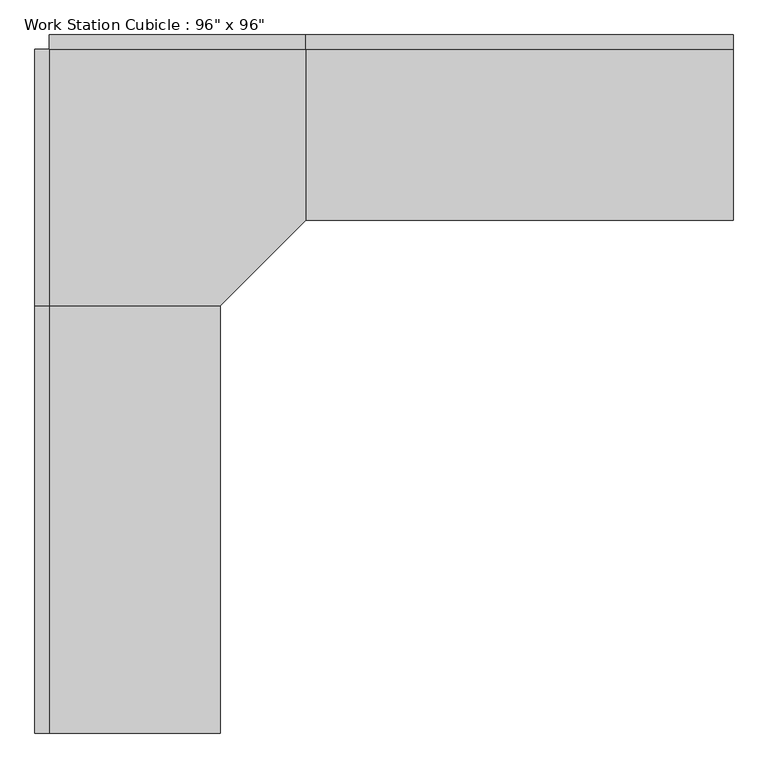
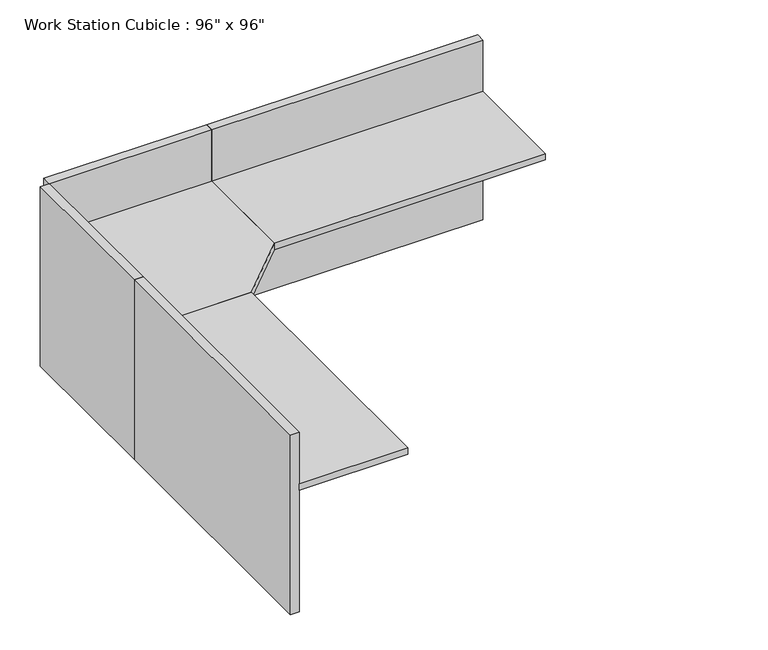
"""IFC4 building model written with IfcOpenShell, lengths in millimetres: furniture geometry."""

from ifc_helpers import new_model, si_unit, frame, origin, origin_with_axes, place, context, project, spatial, polyline, outline, extrude, source, transform, mapped, element, save


def furniture_b89246da(model_context):
    return source(origin(), model_context, "Body", "SweptSolid", [
        extrude(outline(polyline([(-80.9317522, -545.8230076), (833.4682478, -545.8230076), (833.4682478, -1155.4230076), (528.6682478, -1460.2230076), (-80.9317522, -1460.2230076), (-80.9317522, -545.8230076)])), frame((0.0, 0.0, 723.9), z_axis=(0.0, 0.0, 1.0), x_axis=(1.0, 0.0, 0.0)), (0.0, 0.0, 1.0), 38.1),
        extrude(outline(polyline([(528.6682478, -2984.2230076), (-80.9317522, -2984.2230076), (-80.9317522, -1460.2230076), (528.6682478, -1460.2230076), (528.6682478, -2984.2230076)])), frame((0.0, 0.0, 723.9), z_axis=(0.0, 0.0, 1.0), x_axis=(1.0, 0.0, 0.0)), (0.0, 0.0, 1.0), 38.1),
        extrude(outline(polyline([(2357.4682478, -1155.4230076), (833.4682478, -1155.4230076), (833.4682478, -545.8230076), (2357.4682478, -545.8230076), (2357.4682478, -1155.4230076)])), frame((0.0, 0.0, 723.9), z_axis=(0.0, 0.0, 1.0), x_axis=(1.0, 0.0, 0.0)), (0.0, 0.0, 1.0), 38.1),
        extrude(outline(polyline([(2357.4682478, -545.8230076), (833.4682478, -545.8230076), (833.4682478, -495.0230076), (2357.4682478, -495.0230076), (2357.4682478, -545.8230076)])), origin_with_axes(), (0.0, 0.0, 1.0), 1066.8),
        extrude(outline(polyline([(833.4682478, -545.8230076), (-80.9317522, -545.8230076), (-80.9317522, -495.0230076), (833.4682478, -495.0230076), (833.4682478, -545.8230076)])), origin_with_axes(), (0.0, 0.0, 1.0), 1066.8),
        extrude(outline(polyline([(-80.9317522, -1460.2230076), (-131.7317522, -1460.2230076), (-131.7317522, -545.8230076), (-80.9317522, -545.8230076), (-80.9317522, -1460.2230076)])), origin_with_axes(), (0.0, 0.0, 1.0), 1066.8),
        extrude(outline(polyline([(-80.9317522, -2984.2230076), (-131.7317522, -2984.2230076), (-131.7317522, -1460.2230076), (-80.9317522, -1460.2230076), (-80.9317522, -2984.2230076)])), origin_with_axes(), (0.0, 0.0, 1.0), 1066.8),
    ])


if __name__ == "__main__":
    model = new_model("IFC4")
    model_context = context("Model", 3, world=origin())
    ifc_project = project(units=[si_unit("LENGTHUNIT", "METRE", prefix="MILLI")], contexts=[model_context])
    site = spatial("IfcSite", under=ifc_project)
    building = spatial("IfcBuilding", under=site)
    placement = place(None, origin())
    furniture_shape = furniture_b89246da(model_context)
    element("IfcFurniture", 1, ObjectType="Work Station Cubicle : 96\" x 96\"", at=placement, inside=building, context=model_context, shape_type="MappedRepresentation", body=[
        mapped(furniture_shape, transform((0.0, 0.0, 0.0), x_axis=(1.0, 0.0, 0.0), y_axis=(0.0, 1.0, 0.0), z_axis=(0.0, 0.0, 1.0))),
    ])
    save(model, "model.ifc")

# Revit data of these elements
# Type "Work Station Cubicle : 96\" x 96\""
#   Assembly Code = "E2020"
#   Desktop Height = 2' - 6"
#   Desktop1 Width = 2' - 0"
#   Desktop2 Width = 2' - 0"
#   Panel Height = 3' - 6"
#   Panel1 Length = 5' - 0"
#   Panel2 Length = 5' - 0"
#   Cube Panel Material = Textile - Light Gray
#   Work Top Material = Laminate, Ivory, Matte
#   Default Elevation = 0
# Element 1 (IfcFurniture, "Work Station Cubicle : 96\" x 96\"")
#   Materials on its faces: "Textile - Light Gray", "Laminate, Ivory, Matte"
# Materials
#   "Textile - Light Gray": class "Fabric", colour RGB 204 204 204, transparency 0
#   "Laminate, Ivory, Matte": class "Plastic", colour RGB 247 247 239, transparency 0, Description = "Plastic Laminate - Ivory, Matte", Cost = 0
